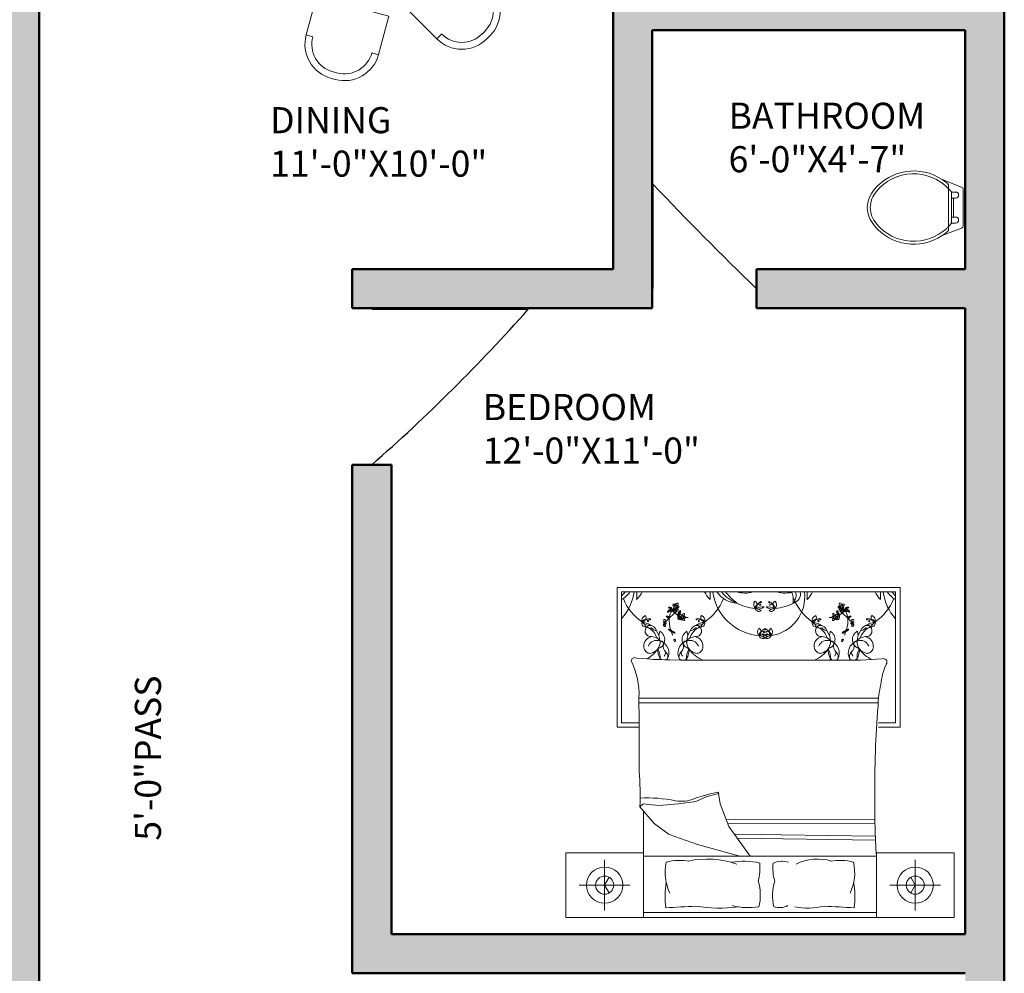
# Model space of a CAD drawing. Units: inches. Extents: x -17 to 536, y -817 to 53.
# Tile 7 of 9: x 268 to 494, y -436 to -217. Entities that reach past the tile are written whole.
import ezdxf

# ---------------------------------------------------------------- set-up
doc = ezdxf.new("R2010")
doc.units = ezdxf.units.IN
doc.header["$MEASUREMENT"] = 0
for name, color, linetype, lineweight in [('A-AREA-IDEN', 7, 'Continuous', 18), ('A-DOOR', 4, 'Continuous', 25), ('A-FLOR-FIXT', 9, 'Continuous', 18), ('A-FURN', 8, 'Continuous', 13), ('A-WALL', 7, 'Continuous', 50), ('A-WALL-PATT', 22, 'Continuous', 13)]:
    doc.layers.add(name, color=color, linetype=linetype, lineweight=lineweight)
doc.styles.get("Standard").update_dxf_attribs({"font": 'arial.ttf'})

# ---------------------------------------------------------------- blocks, each defined once
blk = doc.blocks.new('BED-WITH-NIGHTSTANDS-STANDARD')
for p, q in [((11.79, 75.95), (11.79, 43.78)), ((76.89, 75.95), (11.79, 75.95)), ((12.82, 74.91), (75.86, 74.91)), ((12.82, 44.81), (12.82, 74.91)), ((75.86, 74.91), (75.86, 44.81)), ((76.89, 43.78), (76.89, 75.95)), ((21.62, 65.86), (21.42, 64.85)), ((27.86, 65.86), (28.06, 64.85)), ((60.82, 65.86), (60.62, 64.85)), ((67.06, 65.86), (67.25, 64.85)), ((62.78, 59.23), (26.52, 59.23)), ((71.93, 50.46), (16.83, 50.46)), ((71.85, 49.35), (16.83, 49.35)), ((11.79, 43.78), (16.84, 43.78)), ((16.84, 44.81), (12.82, 44.81)), ((75.86, 44.81), (71.92, 44.81)), ((71.94, 43.78), (76.89, 43.78)), ((32.25, 27.79), (29.9, 26.71)), ((35.15, 28.52), (32.25, 27.79)), ((35.51, 26.17), (35.15, 28.52)), ((17.78, 26.17), (17.06, 25.44)), ((17.06, 25.44), (20.32, 21.65)), ((21.4, 25.8), (17.78, 26.17)), ((25.92, 26.17), (21.4, 25.8)), ((29.9, 26.71), (25.92, 26.17)), ((37.5, 20.92), (35.51, 26.17)), ((17.86, 0), (17.86, 24.51)), ((20.32, 21.65), (23.75, 19.12)), ((71.13, 22.47), (36.86, 22.61)), ((71.12, 21.55), (37.21, 21.69)), ((42.39, 14.11), (37.5, 20.92)), ((23.75, 19.12), (30.26, 16.77)), ((71.17, 18.74), (38.74, 19.2)), ((71.2, 17.82), (39.41, 18.27)), ((30.26, 16.77), (40, 14.11)), ((17.86, 14.11), (71.44, 14.11)), ((8.93, 13.28), (8.93, 1.61)), ((80.37, 13.28), (80.37, 1.61)), ((14.76, 7.44), (3.1, 7.44)), ((74.54, 7.44), (86.21, 7.44)), ((0, 0), (89.3, 0)), ((71.44, 1.15), (17.86, 1.15))]:
    blk.add_line(p, q)
for points in [[(16.87, 33.62, -0.001242), (16.83, 50.56, 0.127202), (15.04, 59.01)], [(71.82, 48.64, -0.056112), (72.47, 53.56, -0.095341), (73.73, 58.29)], [(22.99, 2.23, -0.074897), (23.1, 8.06, 0.472817)], [(44.23, 8.39, -0.14099), (44.41, 2.43, -0.235245)], [(48.05, 8.39, 0.14099), (47.87, 2.43, 0.235245)], [(66.31, 2.23, 0.074897), (66.2, 8.06, -0.472817)]]:
    blk.add_lwpolyline(points, format="xyb")
for points in [[(17.86, 14.88), (0, 14.88), (0, 0)], [(71.44, 0), (71.44, 14.88), (89.3, 14.88), (89.3, 0)], [(8.93, 7.44), (9.97, 9.25)], [(80.37, 7.44), (79.33, 9.25)], [(8.93, 7.44), (9.97, 5.64)], [(80.37, 7.44), (79.33, 5.64)]]:
    blk.add_lwpolyline(points)
for centre, radius in [((25.29, 71.49), 0.227), ((63.39, 71.49), 0.227), ((26.78, 69.09), 0.227), ((61.9, 69.09), 0.227), ((8.93, 7.44), 4.17), ((80.37, 7.44), 4.17), ((8.93, 7.44), 2.08), ((80.37, 7.44), 2.08)]:
    blk.add_circle(centre, radius)
for centre, radius, start, end in [((7.95, 79.1), 7.08, 313.5186, 323.6964), ((9.99, 78.04), 5.68, 299.8884, 326.5383), ((4.14, 76.48), 11.66, 318.1144, 352.255), ((13.17, 76.73), 4.74, 311.0454, 337.4453), ((0.19, 74.18), 16.13, 356.3481, 2.5919), ((36.31, 76.73), 4.74, 202.5547, 228.9546), ((49.3, 74.18), 16.13, 177.4081, 183.6519), ((45.35, 76.48), 11.66, 187.745, 265.5377), ((39.5, 78.04), 5.68, 213.4617, 268.728), ((41.54, 79.1), 7.08, 216.3036, 252.1496), ((45.26, 81.09), 10.53, 215.947, 235.9877), ((41.19, 81.04), 6.41, 252.9798, 286.4569), ((43.73, 84.35), 9.48, 264.3643, 265.6213), ((48.73, 90.84), 16.94, 250.0972, 250.2783), ((45.93, 73.79), 9.03, 278.1803, 7.1364), ((50.46, 81.04), 6.41, 253.5431, 287.0202), ((47.92, 84.35), 9.48, 274.3787, 275.6357), ((42.93, 90.84), 16.94, 289.7217, 289.9028), ((47.1, 72.96), 5.22, 353.3805, 21.883), ((51.89, 74.42), 2.09, 280.9261, 13.6102), ((50.32, 74.13), 2.65, 318.0951, 17.1391), ((39.38, 74.18), 16.13, 356.3481, 2.5919), ((52.37, 76.73), 4.74, 311.0454, 337.4453), ((75.51, 76.73), 4.74, 202.5547, 228.9546), ((88.49, 74.18), 16.13, 177.4081, 183.6519), ((84.54, 76.48), 11.66, 187.745, 221.8856), ((78.69, 78.04), 5.68, 213.4617, 240.1116), ((80.73, 79.1), 7.08, 216.3036, 226.4814), ((24.09, 77.63), 11.66, 201.4092, 235.6135), ((25.39, 77.63), 11.66, 304.3865, 338.5908), ((44.5, 71.97), 1.29, 140.8855, 222.2127), ((43.03, 71.93), 0.974, 301.6373, 61.4609), ((46.34, 70.15), 2.95, 121.989, 161.0841), ((44.85, 72.52), 0.145, 288.4408, 121.989), ((46.81, 72.52), 0.145, 58.011, 251.5592), ((45.32, 70.15), 2.95, 18.9159, 58.011), ((48.62, 71.93), 0.974, 118.5391, 238.3627), ((47.15, 71.97), 1.29, 317.7873, 39.1145), ((63.28, 77.63), 11.66, 201.4092, 235.6135), ((64.59, 77.63), 11.66, 304.3865, 338.5908), ((23.64, 70.33), 0.254, 123.0979, 213.1364), ((24.07, 69.96), 0.687, 92.3172, 160.5201), ((27.22, 64.73), 6.64, 121.1156, 124.8118), ((24, 70.22), 0.592, 82.6008, 147.1845), ((23.83, 71.16), 0.254, 55.6077, 145.6462), ((23.65, 70.61), 0.687, 21.7087, 93.0299), ((20.03, 65.71), 6.64, 53.6254, 57.3216), ((23.92, 70.2), 0.263, 45.7354, 121.1156), ((27.5, 68.52), 3.71, 150.7959, 175.244), ((32.84, 60.63), 12.2, 127.8256, 137.7588), ((23.86, 70.79), 0.592, 342.8042, 79.6943), ((23.81, 70.85), 0.263, 338.2452, 53.6254), ((24.24, 70.68), 0.198, 158.2452, 340.6395), ((24.24, 70.53), 0.198, 225.7354, 48.1297), ((27.97, 72.33), 3.96, 201.7087, 206.2181), ((24.82, 69.63), 1.04, 40.9365, 112.7695), ((24.48, 69.98), 0.61, 49.3812, 95.5456), ((27.5, 68.52), 3.71, 137.5083, 145.9967), ((24.92, 70.22), 0.63, 61.1838, 141.6792), ((27.89, 73.45), 4.45, 220.182, 239.456), ((24.82, 71.92), 0.225, 134.3732, 211.9501), ((25.23, 72.18), 0.717, 211.9501, 255.2442), ((24.83, 71.66), 0.449, 8.5614, 112.5914), ((25.04, 71.17), 0.31, 88.5719, 233.8954), ((25.01, 71.09), 0.223, 228.2946, 6.2474), ((25.35, 71), 0.733, 229.3812, 289.9959), ((24.96, 71.68), 0.151, 352.868, 97.094), ((24.8, 71.35), 0.313, 298.8493, 359.9355), ((24.87, 71.09), 0.358, 4.2123, 48.1587), ((25.6, 71.91), 0.375, 100.9597, 208.7804), ((25.61, 71.14), 0.379, 183.635, 258.4363), ((24.88, 70.1), 0.753, 15.6484, 62.2957), ((25.56, 71.27), 0.217, 178.1325, 268.8919), ((26.01, 71.41), 0.69, 132.3896, 156.5724), ((25.71, 71.32), 0.372, 42.3208, 130.2111), ((25.79, 71.71), 0.47, 226.3462, 279.6513), ((25.29, 72.11), 0.529, 291.6382, 4.947), ((25.3, 70.84), 0.547, 7.4968, 71.2737), ((25.7, 72.2), 0.745, 254.2829, 276.9148), ((25.64, 72.14), 0.174, 4.947, 127.5263), ((25.68, 70.87), 0.176, 215.0752, 14.7644), ((25.31, 70.6), 1.04, 287.889, 359.722), ((25.84, 71.44), 0.196, 279.6513, 42.3208), ((26.61, 69.9), 0.733, 110.6625, 171.2773), ((25.66, 70.27), 0.753, 338.3627, 25.0101), ((44.45, 82.73), 11.66, 242.5854, 265.5377), ((44.5, 71.14), 0.954, 76.148, 182.2415), ((45.99, 63.32), 8.16, 92.7418, 107.407), ((44.3, 72.78), 1.84, 245.6899, 314.4589), ((43.49, 69.11), 1.99, 44.6273, 88.5415), ((44.47, 71.37), 0.967, 196.1963, 296.9726), ((44.7, 71.94), 0.126, 140.0755, 76.148), ((44.87, 72.45), 0.0704, 171.9833, 288.4408), ((45.67, 63.32), 8.16, 72.593, 87.2582), ((47.35, 72.78), 1.84, 225.5411, 294.3101), ((48.16, 69.11), 1.99, 91.4585, 135.3727), ((47.18, 71.37), 0.967, 243.0274, 343.8037), ((46.78, 72.45), 0.0704, 251.5592, 8.0167), ((46.95, 71.89), 0.076, 103.9791, 39.8091), ((47.16, 71.14), 0.954, 357.7585, 103.852), ((47.2, 82.73), 11.66, 274.4623, 297.4146), ((63.02, 70.27), 0.753, 154.9899, 201.6373), ((63.37, 70.6), 1.04, 180.278, 252.111), ((62.07, 69.9), 0.733, 8.7227, 69.3375), ((62.84, 71.44), 0.196, 137.6792, 260.3487), ((62.97, 71.32), 0.372, 49.7889, 137.6792), ((62.89, 71.71), 0.47, 260.3487, 313.6538), ((63.38, 70.84), 0.547, 108.7263, 172.5032), ((63, 70.87), 0.176, 165.2356, 324.9248), ((63.39, 72.11), 0.529, 175.053, 248.3618), ((63.04, 72.14), 0.174, 52.4737, 175.053), ((62.98, 72.2), 0.745, 263.0852, 285.7171), ((60.79, 73.45), 4.45, 300.544, 319.818), ((63.8, 70.1), 0.753, 117.7043, 164.3516), ((63.86, 69.63), 1.04, 67.2305, 139.0635), ((63.33, 71), 0.733, 250.0041, 310.6188), ((63.12, 71.27), 0.217, 271.1081, 1.8675), ((62.67, 71.41), 0.69, 23.4276, 47.6104), ((63.08, 71.91), 0.375, 331.2196, 79.0403), ((63.07, 71.14), 0.379, 281.5637, 356.365), ((55.84, 60.63), 12.2, 42.2412, 52.1744), ((63.85, 71.66), 0.449, 67.4086, 171.4386), ((63.81, 71.09), 0.358, 131.8413, 175.7877), ((63.67, 71.09), 0.223, 173.7526, 311.7054), ((63.75, 70.22), 0.63, 38.3208, 118.8162), ((63.72, 71.68), 0.151, 82.906, 187.132), ((63.88, 71.35), 0.313, 180.0645, 241.1507), ((63.45, 72.18), 0.717, 284.7558, 328.0499), ((63.64, 71.17), 0.31, 306.1046, 91.4281), ((64.2, 69.98), 0.61, 84.4544, 130.6188), ((61.17, 68.52), 3.71, 34.0033, 42.4917), ((63.86, 71.92), 0.225, 328.0499, 45.6268), ((64.81, 70.79), 0.592, 100.3057, 197.1958), ((64.44, 70.53), 0.198, 131.8703, 314.2646), ((64.44, 70.68), 0.198, 199.3605, 21.7548), ((60.71, 72.33), 3.96, 333.7819, 338.2913), ((65.03, 70.61), 0.687, 86.9701, 158.2913), ((61.17, 68.52), 3.71, 4.756, 29.2041), ((64.76, 70.2), 0.263, 58.8844, 134.2646), ((64.86, 70.85), 0.263, 126.3746, 201.7548), ((64.68, 70.22), 0.592, 32.8155, 97.3992), ((64.6, 69.96), 0.687, 19.4799, 87.6828), ((64.85, 71.16), 0.254, 34.3538, 124.3923), ((68.65, 65.71), 6.64, 122.6784, 126.3746), ((61.46, 64.73), 6.64, 55.1882, 58.8844), ((65.04, 70.33), 0.254, 326.8636, 56.9021), ((18.77, 68.29), 1.29, 110.9613, 192.2885), ((18.44, 67.78), 0.967, 166.272, 267.0484), ((17.48, 68.98), 0.974, 271.7131, 31.5367), ((19.45, 65.79), 2.95, 92.0648, 131.1598), ((18.35, 67.57), 0.954, 46.2238, 152.3173), ((15.74, 60.05), 8.16, 62.8176, 77.4827), ((19, 69.09), 1.84, 215.7657, 284.5347), ((16.47, 66.31), 1.99, 14.7031, 58.6173), ((18.92, 68.17), 0.126, 110.2817, 46.2238), ((19.33, 68.52), 0.0704, 142.0591, 258.5166), ((19.35, 68.59), 0.145, 258.5166, 92.0648), ((22.68, 68.16), 0.375, 100.9597, 142.2379), ((22.37, 67.74), 0.227, 273.2768, 86.7232), ((23.09, 67.66), 0.69, 132.3896, 156.5724), ((22.36, 68.36), 0.529, 291.6382, 4.947), ((22.72, 68.39), 0.174, 4.947, 127.5263), ((17.62, 74.63), 8.48, 307.9541, 316.8459), ((23.13, 66.79), 2.52, 82.8698, 91.6736), ((23.48, 69.5), 0.469, 205.5379, 258.6744), ((22.81, 67.91), 1.41, 59.344, 79.7412), ((22.5, 67.92), 1.43, 43.6929, 51.7899), ((23.38, 68.86), 0.429, 355.7131, 81.6568), ((23.14, 68.48), 0.748, 27.3659, 59.344), ((23.71, 68.98), 0.182, 202.5583, 304.2343), ((31.19, 68.33), 7.4, 176.1723, 196.4158), ((25.28, 70.11), 0.61, 305.1128, 351.2773), ((25.59, 68.99), 0.63, 3.8774, 87.1501), ((25.15, 69.23), 0.61, 352.0748, 38.2393), ((25.04, 68.75), 1.04, 343.6301, 55.4631), ((26.48, 69.05), 0.733, 172.0748, 232.6895), ((25.77, 70.21), 0.63, 271.4625, 339.4747), ((25.47, 68.96), 0.753, 318.342, 4.9894), ((26.3, 69.52), 0.225, 134.3732, 211.9501), ((27.89, 73.45), 4.45, 246.1523, 246.9499), ((26.72, 69.78), 0.717, 211.9501, 255.2442), ((26.32, 69.27), 0.449, 8.5614, 112.5914), ((26.53, 68.78), 0.31, 88.5719, 233.8954), ((26.5, 68.69), 0.223, 228.2946, 6.2474), ((26.44, 69.28), 0.151, 352.868, 97.094), ((26.29, 68.96), 0.313, 298.8493, 359.9355), ((26.36, 68.69), 0.358, 4.2123, 48.1587), ((27.09, 69.51), 0.375, 100.9597, 208.7804), ((27.1, 68.74), 0.379, 183.635, 258.4363), ((27.05, 68.88), 0.217, 178.1325, 268.8919), ((27.5, 69.01), 0.69, 132.3896, 156.5724), ((27.19, 68.93), 0.372, 42.3208, 130.2111), ((27.28, 69.31), 0.47, 226.3462, 279.6513), ((26.77, 69.71), 0.529, 291.6382, 4.947), ((26.79, 68.44), 0.547, 7.4968, 71.2737), ((27.19, 69.8), 0.745, 254.2829, 276.9148), ((27.13, 69.74), 0.174, 4.947, 127.5263), ((27.16, 68.47), 0.176, 215.0752, 14.7644), ((27.32, 69.04), 0.196, 279.6513, 42.3208), ((27.89, 73.45), 4.45, 265.2415, 272.8929), ((30.14, 68.59), 0.145, 87.9352, 281.4834), ((30.48, 69.09), 1.84, 255.4653, 324.2343), ((33.75, 60.05), 8.16, 102.5173, 117.1824), ((30.04, 65.79), 2.95, 48.8402, 87.9352), ((30.16, 68.52), 0.0704, 281.4834, 37.9409), ((31.14, 67.57), 0.954, 27.6827, 133.7762), ((30.58, 68.12), 0.076, 133.7729, 69.7333), ((32.01, 68.98), 0.974, 148.4633, 268.2869), ((31.04, 67.78), 0.967, 272.9516, 13.728), ((33.02, 66.31), 1.99, 121.3827, 165.2969), ((30.72, 68.29), 1.29, 347.7115, 69.0387), ((57.96, 68.29), 1.29, 110.9613, 192.2885), ((57.64, 67.78), 0.967, 166.272, 267.0484), ((56.67, 68.98), 0.974, 271.7131, 31.5367), ((58.64, 65.79), 2.95, 92.0648, 131.1598), ((57.54, 67.57), 0.954, 46.2238, 152.3173), ((55.66, 66.31), 1.99, 14.7031, 58.6173), ((58.19, 69.09), 1.84, 215.7657, 284.5347), ((54.93, 60.05), 8.16, 62.8176, 77.4827), ((58.12, 68.17), 0.126, 110.2817, 46.2238), ((58.52, 68.52), 0.0704, 142.0591, 258.5166), ((58.54, 68.59), 0.145, 258.5166, 92.0648), ((60.79, 73.45), 4.45, 267.1071, 274.7585), ((61.36, 69.04), 0.196, 137.6792, 260.3487), ((61.49, 68.93), 0.372, 49.7889, 137.6792), ((61.4, 69.31), 0.47, 260.3487, 313.6538), ((61.52, 68.47), 0.176, 165.2356, 324.9248), ((61.89, 68.44), 0.547, 108.7263, 172.5032), ((61.55, 69.74), 0.174, 52.4737, 175.053), ((61.91, 69.71), 0.529, 175.053, 248.3618), ((61.49, 69.8), 0.745, 263.0852, 285.7171), ((61.63, 68.88), 0.217, 271.1081, 1.8675), ((61.18, 69.01), 0.69, 23.4276, 47.6104), ((61.59, 69.51), 0.375, 331.2196, 79.0403), ((61.58, 68.74), 0.379, 281.5637, 356.365), ((62.36, 69.27), 0.449, 67.4086, 171.4386), ((62.32, 68.69), 0.358, 131.8413, 175.7877), ((62.18, 68.69), 0.223, 173.7526, 311.7054), ((62.23, 69.28), 0.151, 82.906, 187.132), ((62.39, 68.96), 0.313, 180.0645, 241.1507), ((61.96, 69.78), 0.717, 284.7558, 328.0499), ((62.15, 68.78), 0.31, 306.1046, 91.4281), ((62.91, 70.21), 0.63, 200.5253, 268.5375), ((63.21, 68.96), 0.753, 175.0106, 221.658), ((63.08, 68.99), 0.63, 92.8499, 176.1226), ((62.38, 69.52), 0.225, 328.0499, 45.6268), ((60.79, 73.45), 4.45, 293.0501, 293.8477), ((63.64, 68.75), 1.04, 124.5369, 196.3699), ((62.2, 69.05), 0.733, 307.3105, 7.9252), ((63.4, 70.11), 0.61, 188.7227, 234.8872), ((63.53, 69.23), 0.61, 141.7607, 187.9252), ((57.49, 68.33), 7.4, 343.5842, 3.8277), ((65.3, 68.86), 0.429, 98.3432, 184.2869), ((65.53, 68.48), 0.748, 120.656, 152.6341), ((64.97, 68.98), 0.182, 235.7657, 337.4417), ((71.06, 74.63), 8.48, 223.1541, 232.0459), ((66.18, 67.92), 1.43, 128.2101, 136.3071), ((65.87, 67.91), 1.41, 100.2588, 120.656), ((65.55, 66.79), 2.52, 88.3264, 97.1302), ((65.2, 69.5), 0.469, 281.3256, 334.4621), ((65.96, 68.39), 0.174, 52.4737, 175.053), ((66.31, 68.36), 0.529, 175.053, 248.3618), ((65.59, 67.66), 0.69, 23.4276, 47.6104), ((66, 68.16), 0.375, 37.7621, 79.0403), ((66.31, 67.74), 0.227, 93.2768, 266.7232), ((69.33, 68.59), 0.145, 87.9352, 281.4834), ((72.94, 60.05), 8.16, 102.5173, 117.1824), ((69.68, 69.09), 1.84, 255.4653, 324.2343), ((69.23, 65.79), 2.95, 48.8402, 87.9352), ((69.35, 68.52), 0.0704, 281.4834, 37.9409), ((70.33, 67.57), 0.954, 27.6827, 133.7762), ((69.77, 68.12), 0.076, 133.7729, 69.7333), ((71.2, 68.98), 0.974, 148.4633, 268.2869), ((72.21, 66.31), 1.99, 121.3827, 165.2969), ((70.23, 67.78), 0.967, 272.9516, 13.728), ((69.91, 68.29), 1.29, 347.7115, 69.0387), ((19.58, 65.93), 1.34, 109.1312, 279.736), ((19.3, 67.38), 0.821, 216.7319, 296.0245), ((16.92, 62.98), 4.22, 18.2955, 58.7386), ((19.26, 65.53), 1.67, 15.6955, 94.031), ((21.06, 67.75), 1.78, 218.4175, 263.8338), ((16.88, 63.32), 4.79, 3.4924, 33.7117), ((20.52, 63.93), 2.22, 286.8663, 60.0915), ((22.69, 67.39), 0.379, 217.3642, 258.4363), ((22.64, 67.53), 0.217, 178.1325, 268.8919), ((22.78, 67.57), 0.372, 42.3208, 130.2111), ((22.87, 67.96), 0.47, 226.3462, 279.6513), ((22.38, 67.09), 0.547, 7.4968, 71.2737), ((22.78, 68.45), 0.745, 254.2829, 276.9148), ((22.75, 67.12), 0.176, 215.0752, 14.7644), ((22.91, 67.69), 0.196, 279.6513, 42.3208), ((23.66, 63.78), 2.52, 82.8698, 91.6736), ((24.01, 66.5), 0.469, 205.5379, 258.6744), ((23.34, 64.91), 1.41, 59.344, 79.7412), ((23.03, 64.91), 1.43, 43.6929, 51.7899), ((23.91, 65.86), 0.429, 355.7131, 81.6568), ((23.68, 65.48), 0.748, 27.3659, 59.344), ((24.24, 65.97), 0.182, 202.5583, 304.2343), ((31.19, 68.33), 7.4, 200.1059, 206.9968), ((24.57, 65.46), 0.429, 36.5232, 122.4668), ((24.35, 65.08), 0.748, 58.836, 90.8141), ((24.52, 65.8), 0.182, 173.9457, 275.6216), ((24.01, 64.51), 1.41, 38.4388, 58.836), ((22.86, 64.26), 2.52, 26.5064, 35.3102), ((28.97, 63.93), 2.22, 119.9085, 253.1337), ((32.6, 63.32), 4.79, 146.2883, 176.5076), ((32.56, 62.98), 4.22, 121.2614, 161.7045), ((30.23, 65.53), 1.67, 85.969, 164.3045), ((28.42, 67.75), 1.78, 276.1662, 321.5825), ((29.91, 65.93), 1.34, 260.264, 70.8688), ((30.18, 67.38), 0.821, 243.9755, 323.2681), ((45.4, 65.72), 1.29, 140.8855, 222.2127), ((43.93, 65.68), 0.974, 301.6373, 61.4609), ((47.23, 63.9), 2.95, 121.989, 161.0841), ((45.39, 64.89), 0.954, 76.148, 182.2415), ((45.59, 65.7), 0.126, 140.0755, 76.148), ((45.74, 66.28), 0.145, 288.4408, 121.989), ((45.77, 66.21), 0.0704, 171.9833, 288.4408), ((45.91, 66.28), 0.145, 58.011, 251.5592), ((45.89, 66.21), 0.0704, 251.5592, 8.0167), ((46.05, 65.65), 0.076, 103.9791, 39.8091), ((44.43, 63.9), 2.95, 18.9159, 58.011), ((46.26, 64.89), 0.954, 357.7585, 103.852), ((47.73, 65.68), 0.974, 118.5391, 238.3627), ((46.26, 65.72), 1.29, 317.7873, 39.1145), ((58.77, 65.93), 1.34, 109.1312, 279.736), ((58.5, 67.38), 0.821, 216.7319, 296.0245), ((56.12, 62.98), 4.22, 18.2955, 58.7386), ((58.45, 65.53), 1.67, 15.6955, 94.031), ((60.25, 67.75), 1.78, 218.4175, 263.8338), ((56.08, 63.32), 4.79, 3.4924, 33.7117), ((59.71, 63.93), 2.22, 286.8663, 60.0915), ((64.67, 64.51), 1.41, 121.164, 141.5612), ((65.82, 64.26), 2.52, 144.6898, 153.4936), ((64.11, 65.46), 0.429, 57.5332, 143.4768), ((64.33, 65.08), 0.748, 89.1859, 121.164), ((57.49, 68.33), 7.4, 333.0032, 339.8941), ((64.16, 65.8), 0.182, 264.3784, 6.0543), ((64.77, 65.86), 0.429, 98.3432, 184.2869), ((65, 65.48), 0.748, 120.656, 152.6341), ((64.44, 65.97), 0.182, 235.7657, 337.4417), ((65.65, 64.91), 1.43, 128.2101, 136.3071), ((65.34, 64.91), 1.41, 100.2588, 120.656), ((65.02, 63.78), 2.52, 88.3264, 97.1302), ((64.67, 66.5), 0.469, 281.3256, 334.4621), ((65.76, 67.69), 0.196, 137.6792, 260.3487), ((65.89, 67.57), 0.372, 49.7889, 137.6792), ((65.81, 67.96), 0.47, 260.3487, 313.6538), ((66.3, 67.09), 0.547, 108.7263, 172.5032), ((65.92, 67.12), 0.176, 165.2356, 324.9248), ((65.9, 68.45), 0.745, 263.0852, 285.7171), ((68.16, 63.93), 2.22, 119.9085, 253.1337), ((66.04, 67.53), 0.217, 271.1081, 1.8675), ((65.99, 67.39), 0.379, 281.5637, 322.6358), ((71.8, 63.32), 4.79, 146.2883, 176.5076), ((71.76, 62.98), 4.22, 121.2614, 161.7045), ((69.42, 65.53), 1.67, 85.969, 164.3045), ((67.62, 67.75), 1.78, 276.1662, 321.5825), ((69.1, 65.93), 1.34, 260.264, 70.8688), ((69.38, 67.38), 0.821, 243.9755, 323.2681), ((20.07, 62.49), 2.13, 97.1143, 185.0551), ((20.91, 61.68), 2.07, 68.5779, 158.4181), ((18.99, 63.39), 2.69, 283.079, 4.7067), ((19.7, 62.02), 2.59, 35.9599, 87.6409), ((24.57, 61.5), 3.44, 143.6555, 147.2989), ((21.92, 63), 0.554, 344.8529, 102.6959), ((20.86, 60.85), 2.85, 330.8249, 70.7178), ((24.16, 64.24), 1.43, 66.3901, 74.4871), ((25.09, 65.85), 0.469, 219.5056, 272.6421), ((25, 63.84), 0.172, 79.5616, 257.2949), ((24.98, 63.73), 0.28, 259.5864, 79.5616), ((28.63, 60.85), 2.85, 109.2822, 209.1751), ((27.56, 63), 0.554, 77.3041, 195.1471), ((29.79, 62.02), 2.59, 92.3591, 144.0401), ((24.91, 61.5), 3.44, 32.7011, 36.3445), ((30.5, 63.39), 2.69, 175.2933, 256.921), ((28.58, 61.68), 2.07, 21.5819, 111.4221), ((29.42, 62.49), 2.13, 354.9449, 82.8857), ((45.2, 66.54), 1.84, 245.6899, 314.4589), ((46.88, 57.07), 8.16, 92.7418, 107.407), ((45.37, 65.13), 0.967, 196.1963, 296.9726), ((44.39, 62.86), 1.99, 44.6273, 88.5415), ((46.46, 66.54), 1.84, 225.5411, 294.3101), ((44.78, 57.07), 8.16, 72.593, 87.2582), ((46.29, 65.13), 0.967, 243.0274, 343.8037), ((47.27, 62.86), 1.99, 91.4585, 135.3727), ((59.26, 62.49), 2.13, 97.1143, 185.0551), ((60.1, 61.68), 2.07, 68.5779, 158.4181), ((58.18, 63.39), 2.69, 283.079, 4.7067), ((58.89, 62.02), 2.59, 35.9599, 87.6409), ((63.77, 61.5), 3.44, 143.6555, 147.2989), ((61.11, 63), 0.554, 344.8529, 102.6959), ((60.05, 60.85), 2.85, 330.8249, 70.7178), ((63.7, 63.73), 0.28, 100.4384, 280.4136), ((63.59, 65.85), 0.469, 267.3579, 320.4944), ((63.68, 63.84), 0.172, 282.7051, 100.4384), ((64.52, 64.24), 1.43, 105.5129, 113.6099), ((67.82, 60.85), 2.85, 109.2822, 209.1751), ((66.76, 63), 0.554, 77.3041, 195.1471), ((68.98, 62.02), 2.59, 92.3591, 144.0401), ((64.11, 61.5), 3.44, 32.7011, 36.3445), ((69.69, 63.39), 2.69, 175.2933, 256.921), ((67.77, 61.68), 2.07, 21.5819, 111.4221), ((68.61, 62.49), 2.13, 354.9449, 82.8857), ((19.45, 62.27), 1.51, 178.9462, 275.5144), ((15.52, 65.52), 6.76, 296.7003, 326.3329), ((24.57, 61.5), 3.44, 175.2696, 214.215), ((17.99, 59.89), 3.7, 350.8446, 31.1782), ((24.22, 62.38), 1.83, 164.8529, 228.4347), ((25.26, 62.38), 1.83, 311.5653, 15.1471), ((24.91, 61.5), 3.44, 325.785, 4.7304), ((31.49, 59.89), 3.7, 148.8218, 190.2867), ((33.97, 65.52), 6.76, 213.6671, 248.5059), ((30.03, 62.27), 1.51, 264.4856, 1.0538), ((58.65, 62.27), 1.51, 178.9462, 275.5144), ((54.71, 65.52), 6.76, 291.4941, 326.3329), ((63.77, 61.5), 3.44, 175.2696, 214.215), ((57.19, 59.89), 3.7, 349.7133, 31.1782), ((63.42, 62.38), 1.83, 164.8529, 228.4347), ((64.46, 62.38), 1.83, 311.5653, 15.1471), ((64.11, 61.5), 3.44, 325.785, 4.7304), ((70.68, 59.89), 3.7, 148.8218, 190.751), ((73.16, 65.52), 6.76, 213.6671, 246.3547), ((69.23, 62.27), 1.51, 264.4856, 1.0538), ((15.86, 58.95), 0.824, 62.6588, 176.02), ((25.46, 152.19), 92.96, 264.3113, 270.6567), ((22.58, 60.22), 1.08, 217.675, 239.9707), ((20.43, 61.37), 2.57, 330.0851, 352.564), ((22.12, 60.01), 1.34, 336.1646, 48.4347), ((22.58, 60.22), 1.08, 296.442, 315.5483), ((27.36, 60.01), 1.34, 131.5653, 203.8354), ((26.91, 60.22), 1.08, 224.4517, 246.771), ((29.06, 61.37), 2.57, 187.436, 209.9149), ((26.91, 60.22), 1.08, 293.2856, 322.325), ((61.77, 60.22), 1.08, 217.675, 246.7144), ((59.62, 61.37), 2.57, 330.0851, 352.564), ((61.77, 60.22), 1.08, 293.2856, 315.5483), ((61.32, 60.01), 1.34, 336.1646, 48.4347), ((65.51, 146.09), 86.9, 268.1965, 274.7598), ((66.56, 60.01), 1.34, 131.5653, 203.8354), ((66.1, 60.22), 1.08, 224.4517, 253.3657), ((68.25, 61.37), 2.57, 187.436, 209.9149), ((66.1, 60.22), 1.08, 287.4186, 322.325), ((73.05, 58.74), 0.814, 326.1736, 113.4781), ((280.38, 30.86), 209.31, 175.1265, 180.8855), ((-64.82, 27.66), 81.91, 358.447, 4.1706), ((18.59, -6.18), 33.7, 78.6608, 92.5481), ((26.65, 33.99), 7.27, 258.6608, 293.7384), ((41.35, -5.23), 34.63, 100.6617, 109.8806), ((34.95, 28.59), 0.215, 340.2464, 91.1377), ((231.53, 25.03), 160.46, 179.0718, 183.9), ((34.37, 10.4), 11.51, 168.2417, 204.8684), ((26.18, 1.18), 11.97, 78.9631, 104.8961), ((32.48, -7.33), 20.76, 70.7385, 101.9603), ((40.88, -2.79), 15.75, 76.3762, 100.1383), ((33.71, 11.37), 10.94, 344.1707, 5.9871), ((58.57, 11.37), 10.94, 174.0129, 195.8293), ((49.69, 8.22), 4.73, 71.4593, 114.9817), ((57.96, 2.06), 11.37, 73.8254, 116.1239), ((63.13, 1.18), 11.97, 75.1039, 101.0369), ((54.94, 10.4), 11.51, 335.1316, 11.7583), ((72.21, -847.63), 851.28, 92.85022, 93.31479), ((35.23, 34.54), 32.39, 260.503, 277.7804), ((42.07, 18.17), 15.91, 256.04, 278.4751), ((49.09, 6.68), 4.42, 253.8974, 296.6563), ((55.71, 17.85), 15.7, 258.8159, 283.6573), ((17.09, -847.63), 851.28, 86.68521, 87.14978)]:
    blk.add_arc(centre, radius, start, end)
blk = doc.blocks.new('WC-22IN')
for p, q in [((18.71, 12.76), (18.71, 13.68)), ((18.71, 12.76), (18.71, 8.42)), ((18.71, 4.08), (18.71, 8.42)), ((18.71, 3.16), (18.71, 4.08))]:
    blk.add_line(p, q)
for points in [[(17.19, 14.88, 0.383919), (1.59, 12.57, 0.163732), (0, 8.42, 0.359733)], [(18.71, 12.76, 0.448546), (2.1, 12.15, 0.162618), (0.66, 8.42, 0.470877)], [(18.71, 13.68, 0.040937), (17.19, 14.88, 0.163732)], [(22.05, 8.42), (22.05, 12.63, 0.31031), (21.69, 13.15), (17.19, 14.88, 0.209071)], [(19.37, 12, 0.022712), (18.71, 12.76, 0.162618)], [(19.37, 8.42), (19.37, 12, 0.476108)], [(19.37, 12), (20.3, 12, -1), (20.3, 10.59), (19.82, 10.59)], [(17.19, 1.97, -0.383919), (1.59, 4.28, -0.163732), (0, 8.42, -0.359733)], [(18.26, 3.64, -0.431639), (2.1, 4.7, -0.162618), (0.66, 8.42, -0.470877)], [(22.05, 8.42), (22.05, 4.21, -0.31031), (21.69, 3.7), (17.19, 1.97, -0.209071)], [(19.37, 8.42), (19.37, 4.85, -0.022712)], [(19.37, 4.85, -0.022712), (18.71, 4.08, -0.162618)], [(19.37, 4.85), (20.3, 4.85, 1), (20.3, 6.25), (19.82, 6.25)], [(18.71, 3.16, -0.040937), (17.19, 1.97, -0.163732)], [(18.71, 4.08, -0.014165), (18.26, 3.64, -0.162618)]]:
    blk.add_lwpolyline(points, format="xyb")
for points in [[(19.82, 10.59), (19.37, 10.59)], [(19.82, 10.59), (19.82, 6.25)], [(19.82, 6.25), (19.37, 6.25)]]:
    blk.add_lwpolyline(points)
blk = doc.blocks.new('DINING-CHAIR-COMPACT')
for p, q in [((8.8, 19.04), (0, 16.68)), ((9.29, 17.47), (8.86, 19.06)), ((4.47, 0), (0, 16.68)), ((17.52, 11.95), (17.28, 12.86)), ((19.04, 12.35), (18.79, 13.26)), ((13.27, 2.36), (4.47, 0)), ((12.86, 3.87), (13.27, 2.36))]:
    blk.add_line(p, q)
for centre, radius, start, end in [((10.91, 11.15), 8.16, 15, 105), ((10.91, 11.15), 6.59, 15, 105), ((11.15, 10.24), 6.59, 285, 15), ((11.15, 10.24), 8.16, 285, 15)]:
    blk.add_arc(centre, radius, start, end)

msp = doc.modelspace()

# ---------------------------------------------------------------- hatches: boundary and pattern name
at = {"layer": 'A-WALL-PATT'}
h = msp.add_hatch(color=256, dxfattribs=at)
h.dxf.hatch_style = 1
h.paths.add_polyline_path([(217.37, -544.45), (208.37, -544.45), (208.37, -775.45), (217.37, -775.45)], flags=17)
h.paths.add_polyline_path([(327.37, -544.45), (318.37, -544.45), (318.37, -775.45), (327.37, -775.45)], flags=17)
h.paths.add_polyline_path([(494.37, 11.55), (41.37, 11.55), (41.37, -775.45), (50.37, -775.45), (50.37, -739.45), (184.37, -739.45), (184.37, -730.45), (50.37, -730.45), (50.37, -610.45), (172.37, -610.45), (172.37, -601.45), (155.37, -601.45), (155.37, -577.45), (146.37, -577.45), (146.37, -601.45), (50.37, -601.45), (50.37, -553.45), (172.37, -553.45), (172.37, -544.45), (50.37, -544.45), (50.37, -436.45), (191.37, -436.45), (191.37, -319.45), (182.37, -319.45), (182.37, -427.45), (50.37, -427.45), (50.37, -283.45), (98.37, -283.45), (98.37, -274.45), (50.37, -274.45), (50.37, -219.45), (122.37, -219.45), (122.37, -283.45), (191.37, -283.45), (191.37, -274.45), (131.37, -274.45), (131.37, -219.45), (131.37, -150.45), (146.37, -150.45), (146.37, -141.45), (122.37, -141.45), (122.37, -210.45), (50.37, -210.45), (50.37, -150.45), (98.37, -150.45), (98.37, -141.45), (50.37, -141.45), (50.37, 2.55), (182.37, 2.55), (182.37, -150.45), (191.37, -150.45), (191.37, 2.55), (263.37, 2.55), (263.37, -141.45), (227.37, -141.45), (227.37, -150.45), (263.37, -150.45), (263.37, -553.45), (272.37, -553.45), (272.37, -150.45), (308.37, -150.45), (308.37, -141.45), (272.37, -141.45), (272.37, 2.55), (344.37, 2.55), (344.37, -150.45), (353.37, -150.45), (353.37, 2.55), (485.37, 2.55), (485.37, -141.45), (437.37, -141.45), (437.37, -150.45), (485.37, -150.45), (485.37, -210.45), (413.37, -210.45), (413.37, -141.45), (389.37, -141.45), (389.37, -150.45), (404.37, -150.45), (404.37, -219.45), (404.37, -274.45), (353.37, -274.45), (344.37, -274.45), (344.37, -283.45), (353.37, -283.45), (413.37, -283.45), (413.37, -219.45), (485.37, -219.45), (485.37, -274.45), (437.37, -274.45), (437.37, -283.45), (485.37, -283.45), (485.37, -427.45), (353.37, -427.45), (353.37, -319.45), (344.37, -319.45), (344.37, -436.45), (485.37, -436.45), (485.37, -544.45), (363.37, -544.45), (363.37, -553.45), (485.37, -553.45), (485.37, -601.45), (389.37, -601.45), (389.37, -577.45), (380.37, -577.45), (380.37, -601.45), (363.37, -601.45), (363.37, -610.45), (485.37, -610.45), (485.37, -730.45), (351.37, -730.45), (351.37, -739.45), (485.37, -739.45), (485.37, -775.45), (494.37, -775.45)])

# ---------------------------------------------------------------- linework, layer by layer
at = {"layer": 'A-DOOR'}
for p, q in [((413.6, -278.95), (413.6, -254.95)), ((413.6, -278.95), (413.37, -278.95)), ((348.87, -283.68), (348.87, -283.45)), ((348.87, -283.68), (384.87, -283.68))]:
    msp.add_line(p, q, dxfattribs=at)
for centre, radius, start, end in [((926.45, 229.04), 705.17, 223.34179, 226.08616), ((81.69, -14.6), 405.36, 311.2317, 318.4101)]:
    msp.add_arc(centre, radius, start, end, dxfattribs=at)
at = {"layer": 'A-WALL'}
for p, q in [((494.37, 11.55), (494.37, -775.45)), ((272.37, -150.45), (272.37, -553.45)), ((404.37, -150.45), (404.37, -219.45)), ((404.37, -219.45), (404.37, -274.45)), ((413.37, -219.45), (485.37, -219.45)), ((413.37, -219.45), (413.37, -283.45)), ((485.37, -219.45), (485.37, -274.45)), ((344.37, -274.45), (344.37, -283.45)), ((344.37, -274.45), (353.37, -274.45)), ((353.37, -274.45), (404.37, -274.45)), ((437.37, -274.45), (437.37, -283.45)), ((437.37, -274.45), (485.37, -274.45)), ((344.37, -283.45), (353.37, -283.45)), ((353.37, -283.45), (413.37, -283.45)), ((437.37, -283.45), (485.37, -283.45)), ((485.37, -283.45), (485.37, -427.45)), ((353.37, -319.45), (344.37, -319.45)), ((344.37, -319.45), (344.37, -436.45)), ((353.37, -319.45), (353.37, -427.45)), ((353.37, -427.45), (485.37, -427.45)), ((344.37, -436.45), (485.37, -436.45))]:
    msp.add_line(p, q, dxfattribs=at)

# ---------------------------------------------------------------- block references
at = {"layer": 'A-FLOR-FIXT'}
msp.add_blockref('WC-22IN', (462.85, -268.72), dxfattribs=at)
at = {"layer": 'A-FURN'}
for p, rotation in [((355.13, -211.17), 300.0000000082552), ((338.35, -207.92), 239.999999980094)]:
    msp.add_blockref('DINING-CHAIR-COMPACT', p, dxfattribs=dict(at, rotation=rotation))
msp.add_blockref('BED-WITH-NIGHTSTANDS-STANDARD', (393.5, -423.61), dxfattribs=at)

# ---------------------------------------------------------------- texts
at = {"layer": 'A-AREA-IDEN', "char_height": 6, "attachment_point": 1}
for s, insert in [('DINING\\P11\'-0"X10\'-0"', (325.48, -237.19)), ('BATHROOM\\P6\'-0"X4\'-7"', (430.94, -236.17)), ('BEDROOM\\P12\'-0"X11\'-0"', (374.39, -303.2))]:
    msp.add_mtext(s, dxfattribs=dict(at, insert=insert))
at = {"layer": 'A-AREA-IDEN', "insert": (294.36, -405.94), "char_height": 6, "attachment_point": 1, "rotation": 90}
msp.add_mtext('5\'-0"PASS', dxfattribs=at)

doc.saveas('drawing.dxf')
